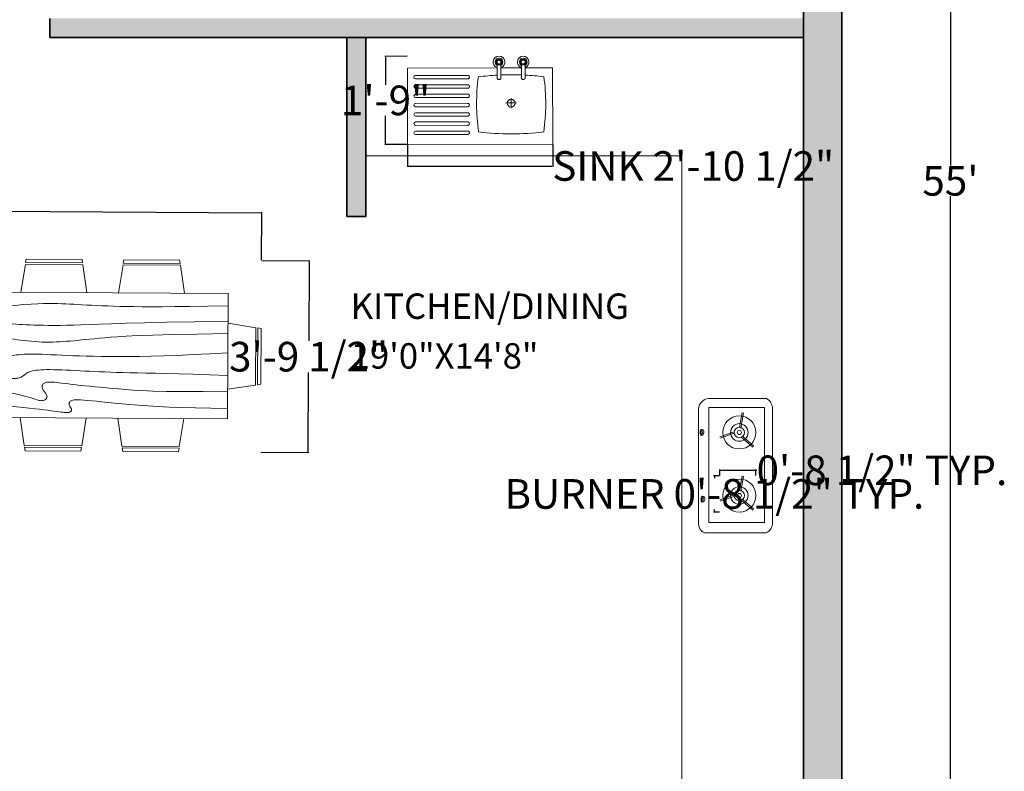
# Model space of a CAD drawing. Units: inches. Extents: x 1319 to 2030, y 219 to 1069.
# Tile 23 of 28: x 1776 to 2008, y 486 to 663. Entities that reach past the tile are written whole.
import ezdxf

# ---------------------------------------------------------------- set-up
doc = ezdxf.new("R2010")
doc.units = ezdxf.units.IN
doc.header["$MEASUREMENT"] = 0
doc.layers.get('0').update_dxf_attribs({"color": 12})
for name, color, linetype, lineweight in [('A-ANNO-DIMS', 2, 'Continuous', 18), ('A-AREA-IDEN', 250, 'Continuous', 18), ('A-EQPM', 8, 'Continuous', 18), ('A-FLOR-CASE', 8, 'Continuous', 18), ('A-WALL-PATT', 252, 'Continuous', 13), ('C-PROP', 7, 'Continuous', 35), ('furniture', 250, 'Continuous', 18), ('PLUMBING FIXTURES', 252, 'Continuous', 18), ('walls', 250, 'Continuous', 35)]:
    doc.layers.add(name, color=color, linetype=linetype, lineweight=lineweight)
doc.styles.get("Standard").update_dxf_attribs({"font": 'arial.ttf'})
doc.dimstyles.get("Standard").update_dxf_attribs({"dimtxt": 7, "dimasz": 0.18, "dimexe": 0.18, "dimexo": 0.0625, "dimgap": 0.09, "dimtad": 0, "dimtih": 1, "dimtoh": 1, "dimzin": 0, "dimdsep": 46, "dimlunit": 3, "dimtxsty": 'Standard', "dimcen": 0.09, "dimadec": 0, "dimazin": 0, "dimtfac": 1, "dimtofl": 0, "dimtmove": 0, "dimatfit": 3, "dimfxl": 1, "dimtolj": 1, "dimtzin": 0, "dimarcsym": 0})

# ---------------------------------------------------------------- blocks, each defined once
blk = doc.blocks.new('Dining Set - 36 x 72 in.')
for p, q in [((-22.2343, 26.00059), (-23.4847, 17.99762)), ((-22.2304, 26), (-5.7608, 26)), ((-22, 27.5), (-22.1562, 26.50042)), ((-5.8416, 26.5), (-22.1534, 26.5)), ((-22, 27.5), (-6, 27.5)), ((-5.8437, 26.49966), (-6, 27.5)), ((-4.5152, 17.99762), (-5.7655, 25.99926)), ((5.7657, 26.00059), (4.5153, 17.99762)), ((5.7696, 26), (22.2392, 26)), ((6, 27.5), (5.8438, 26.50042)), ((22.1584, 26.5), (5.8466, 26.5)), ((6, 27.5), (22, 27.5)), ((22.1563, 26.49966), (22, 27.5)), ((23.4848, 17.99762), (22.2345, 25.99926)), ((36, 18), (-36, 18)), ((-36, 18), (-36, -18)), ((36, -18), (36, 18)), ((-44.0006, 8.23428), (-35.9976, 9.48474)), ((44.0006, 8.23428), (35.9976, 9.48474)), ((-45.5, 8), (-44.5004, 8.15617)), ((-45.5, 8), (-45.5, -8)), ((-44.5, -8.15843), (-44.5, 8.15338)), ((-44, 8.23041), (-44, -8.23915)), ((44, 8.23041), (44, -8.23915)), ((44.5, -8.15843), (44.5, 8.15338)), ((45.5, 8), (44.5005, 8.15617)), ((45.5, 8), (45.5, -8)), ((-44.4997, -8.15631), (-45.5, -8)), ((-35.9976, -9.48476), (-43.9993, -8.2345)), ((35.9976, -9.48476), (43.9993, -8.2345)), ((44.4997, -8.15631), (45.5, -8)), ((-36, -18), (36, -18)), ((-22.2343, -26.0006), (-23.4847, -17.99762)), ((-4.5152, -17.99762), (-5.7655, -25.99928)), ((5.7657, -26.0006), (4.5153, -17.99762)), ((23.4848, -17.99762), (22.2345, -25.99928)), ((-22.2304, -26), (-5.7608, -26)), ((-22, -27.5), (-22.1562, -26.50044)), ((-5.8416, -26.5), (-22.1534, -26.5)), ((-22, -27.5), (-6, -27.5)), ((-5.8437, -26.49967), (-6, -27.5)), ((5.7696, -26), (22.2392, -26)), ((6, -27.5), (5.8438, -26.50044)), ((22.1584, -26.5), (5.8466, -26.5)), ((6, -27.5), (22, -27.5)), ((22.1563, -26.49967), (22, -27.5))]:
    blk.add_line(p, q)
for points in [[(-36, 15), (-31.1772, 14.97754), (-26.8079, 14.91406), (-22.8538, 14.81543), (-19.276, 14.6875), (-16.0362, 14.53613), (-13.0957, 14.36718), (-10.4159, 14.18652), (-7.9583, 14), (-5.6904, 13.81315), (-3.6035, 13.63021), (-1.6954, 13.45508), (0.0365, 13.29166), (1.5945, 13.14388), (2.9811, 13.01562), (4.1988, 12.9108), (5.25, 12.83333), (6.1393, 12.78613), (6.8802, 12.76823), (7.4883, 12.77767), (7.9792, 12.8125), (8.3685, 12.87077), (8.6719, 12.95052), (8.9049, 13.0498), (9.0833, 13.16666), (9.2205, 13.29899), (9.3216, 13.44401), (9.3895, 13.59879), (9.4271, 13.76041), (9.4373, 13.92594), (9.4232, 14.09245), (9.3875, 14.257), (9.3333, 14.41666), (9.2638, 14.56917), (9.1836, 14.71484), (9.0975, 14.85465), (9.0104, 14.98958), (8.9272, 15.1206), (8.8529, 15.2487), (8.7922, 15.37483), (8.75, 15.5), (8.7305, 15.62467), (8.7344, 15.74739), (8.7617, 15.86621), (8.8125, 15.97916), (8.8867, 16.08431), (8.9844, 16.17968), (9.1055, 16.26334), (9.25, 16.33333), (9.4189, 16.38802), (9.6172, 16.42708), (9.8506, 16.45052), (10.125, 16.45833), (10.4463, 16.45052), (10.8203, 16.42708), (11.2529, 16.38802), (11.75, 16.33333), (12.3184, 16.26318), (12.9694, 16.17838), (13.7151, 16.07991), (14.5677, 15.96875), (15.5395, 15.84586), (16.6426, 15.71224), (17.8893, 15.56884), (19.2917, 15.41666), (20.859, 15.25667), (22.5879, 15.08984), (24.4721, 14.91715), (26.5052, 14.73958), (28.6809, 14.5581), (30.9929, 14.3737), (33.4347, 14.18733), (36, 14)], [(-36, 10), (-28.9766, 10.14274), (-23.1725, 10.20442), (-18.4241, 10.19775), (-14.5677, 10.13541), (-11.4399, 10.03011), (-8.877, 9.89453), (-6.7154, 9.74137), (-4.7917, 9.58333), (-2.9698, 9.43082), (-1.2246, 9.28515), (0.4415, 9.14534), (2.026, 9.01041), (3.5266, 8.87939), (4.9408, 8.7513), (6.266, 8.62516), (7.5, 8.5), (8.6411, 8.37549), (9.6914, 8.2539), (10.6538, 8.13818), (11.5312, 8.03125), (12.3267, 7.93603), (13.043, 7.85547), (13.6831, 7.79248), (14.25, 7.75), (14.7471, 7.7303), (15.1797, 7.73307), (15.5537, 7.75732), (15.875, 7.80208), (16.1494, 7.86637), (16.3828, 7.94922), (16.5811, 8.04964), (16.75, 8.16666), (16.8944, 8.29915), (17.0143, 8.44531), (17.1089, 8.60319), (17.1771, 8.77083), (17.218, 8.94629), (17.2305, 9.1276), (17.2137, 9.31282), (17.1667, 9.5), (17.0895, 9.6875), (16.987, 9.875), (16.8649, 10.0625), (16.7292, 10.25), (16.5856, 10.4375), (16.4401, 10.625), (16.2985, 10.8125), (16.1667, 11), (16.05, 11.18733), (15.9518, 11.3737), (15.8752, 11.5581), (15.8229, 11.73958), (15.798, 11.91715), (15.8034, 12.08984), (15.842, 12.25667), (15.9167, 12.41666), (16.0295, 12.56836), (16.1784, 12.70833), (16.3605, 12.83268), (16.5729, 12.9375), (16.8127, 13.01888), (17.0768, 13.07291), (17.3625, 13.0957), (17.6667, 13.08333), (17.9894, 13.03312), (18.3418, 12.94726), (18.7382, 12.82918), (19.1927, 12.68229), (19.7195, 12.51001), (20.3327, 12.31575), (21.0465, 12.10294), (21.875, 11.875), (22.8357, 11.63354), (23.959, 11.37304), (25.2786, 11.08618), (26.8282, 10.76562), (28.6414, 10.40405), (30.752, 9.99414), (33.1936, 9.52856), (36, 9)], [(-36, 5.5), (-30.7157, 5.3348), (-26.069, 5.20963), (-21.9946, 5.11767), (-18.4271, 5.05208), (-15.3009, 5.00602), (-12.5508, 4.97265), (-10.1112, 4.94515), (-7.9167, 4.91666), (-5.909, 4.88167), (-4.0586, 4.83984), (-2.3429, 4.79215), (-0.7396, 4.73958), (0.7739, 4.6831), (2.22, 4.6237), (3.6213, 4.56233), (5, 4.5), (6.373, 4.43782), (7.7344, 4.3776), (9.0723, 4.32129), (10.375, 4.27083), (11.6309, 4.22819), (12.8281, 4.19531), (13.9551, 4.17415), (15, 4.16666), (15.954, 4.17448), (16.819, 4.19791), (17.6001, 4.23698), (18.3021, 4.29166), (18.9299, 4.36198), (19.4883, 4.44791), (19.9823, 4.54948), (20.4167, 4.66666), (20.7969, 4.79899), (21.1302, 4.94401), (21.4245, 5.09879), (21.6875, 5.26041), (21.9271, 5.42594), (22.1511, 5.59245), (22.3672, 5.757), (22.5834, 5.91666), (22.8065, 6.06868), (23.0404, 6.21093), (23.2879, 6.34147), (23.5521, 6.45833), (23.8358, 6.55957), (24.142, 6.64323), (24.4735, 6.70735), (24.8334, 6.75), (25.2235, 6.76969), (25.642, 6.76692), (26.0858, 6.74267), (26.5521, 6.69791), (27.0379, 6.63362), (27.5404, 6.55078), (28.0565, 6.45036), (28.5834, 6.33333), (29.1242, 6.19987), (29.7071, 6.04687), (30.3661, 5.87044), (31.1354, 5.66666), (32.0493, 5.43164), (33.142, 5.16146), (34.4475, 4.85221), (36, 4.5)], [(-36, -1), (-30.7915, -0.6591), (-26.0195, -0.38216), (-21.6519, -0.16284), (-17.6563, 0.00521), (-14.0005, 0.12833), (-10.6523, 0.21289), (-7.5796, 0.26522), (-4.75, 0.29166), (-2.134, 0.29793), (0.2878, 0.28711), (2.5317, 0.26163), (4.6146, 0.22396), (6.5529, 0.17651), (8.3633, 0.12174), (10.0623, 0.06209), (11.6667, 0), (13.1899, -0.06201), (14.6341, -0.1211), (15.9982, -0.17432), (17.2813, -0.21875), (18.4823, -0.25147), (19.6003, -0.26953), (20.6343, -0.27002), (21.5834, -0.25), (22.4481, -0.20768), (23.2357, -0.14584), (23.9549, -0.06836), (24.6146, 0.02083), (25.2235, 0.11784), (25.7904, 0.21875), (26.3241, 0.31966), (26.8334, 0.41666), (27.3265, 0.50618), (27.8099, 0.58593), (28.2894, 0.65397), (28.7709, 0.70833), (29.2601, 0.74707), (29.763, 0.76823), (30.2855, 0.76985), (30.8334, 0.75), (31.4088, 0.70784), (31.9994, 0.64713), (32.589, 0.57275), (33.1615, 0.48958), (33.7008, 0.4025), (34.1908, 0.3164), (34.6153, 0.23616), (34.9584, 0.16666), (35.2099, 0.11165), (35.3848, 0.07031), (35.504, 0.04069), (35.5886, 0.02083), (35.6594, 0.00879), (35.7377, 0.0026), (35.8442, 0.00032), (36, 0)], [(-36, -6.5), (-27.1843, -6.31267), (-20.084, -6.1263), (-14.469, -5.9419), (-10.1094, -5.76042), (-6.7752, -5.58285), (-4.2363, -5.41016), (-2.2629, -5.24333), (-0.625, -5.08334), (0.8708, -4.93099), (2.2715, -4.78646), (3.5872, -4.64974), (4.8281, -4.52084), (6.0046, -4.39974), (7.127, -4.28646), (8.2053, -4.18099), (9.25, -4.08334), (10.2705, -3.99382), (11.2734, -3.91407), (12.2647, -3.84603), (13.25, -3.79167), (14.2354, -3.75293), (15.2266, -3.73177), (16.2295, -3.73015), (17.25, -3.75), (18.2912, -3.79248), (19.3451, -3.85547), (20.4009, -3.93604), (21.4479, -4.03125), (22.4754, -4.13819), (23.4727, -4.25391), (24.4289, -4.37549), (25.3334, -4.5), (26.1785, -4.62492), (26.9694, -4.74935), (27.7145, -4.87281), (28.4219, -4.99479), (29.1, -5.11483), (29.7572, -5.23242), (30.4016, -5.34709), (31.0417, -5.45834), (31.6837, -5.56437), (32.3262, -5.65821), (32.9658, -5.73153), (33.599, -5.77604), (34.2224, -5.78345), (34.8327, -5.74545), (35.4264, -5.65373), (36, -5.5)], [(-36, -10), (-26.4022, -9.81299), (-18.4675, -9.62891), (-11.9839, -9.45069), (-6.7396, -9.28125), (-2.5226, -9.12354), (0.8789, -8.98047), (3.6769, -8.85498), (6.0833, -8.75), (8.2767, -8.66765), (10.3021, -8.60677), (12.1712, -8.56543), (13.8958, -8.54167), (15.4876, -8.53353), (16.9583, -8.53907), (18.3197, -8.55632), (19.5834, -8.58334), (20.7616, -8.61841), (21.8685, -8.66081), (22.9188, -8.71004), (23.9271, -8.76563), (24.9081, -8.82707), (25.8763, -8.89388), (26.8465, -8.96558), (27.8334, -9.04167), (28.8474, -9.12118), (29.8828, -9.20117), (30.93, -9.27824), (31.9792, -9.34896), (33.0205, -9.40991), (34.0443, -9.45768), (35.0407, -9.48885), (36, -9.5)], [(-36, -14.5), (-30.0881, -14.33513), (-25.0332, -14.21224), (-20.7312, -14.12647), (-17.0781, -14.07292), (-13.97, -14.04671), (-11.3027, -14.04297), (-8.9724, -14.05681), (-6.875, -14.08334), (-4.9224, -14.11833), (-3.0905, -14.16016), (-1.3709, -14.20785), (0.2448, -14.26042), (1.7647, -14.3169), (3.1973, -14.3763), (4.5507, -14.43767), (5.8333, -14.5), (7.0554, -14.5621), (8.235, -14.62175), (9.3922, -14.67652), (10.5469, -14.72396), (11.7192, -14.76164), (12.929, -14.78711), (14.1965, -14.79794), (15.5417, -14.79167), (16.9933, -14.76424), (18.6152, -14.70508), (20.4804, -14.60197), (22.6615, -14.44271), (25.2312, -14.21509), (28.2624, -13.9069), (31.8277, -13.50594), (36, -13)]]:
    blk.add_lwpolyline(points)
blk = doc.blocks.new('dining area')
at = {"layer": 'furniture', "xscale": 0.6659924291999282, "yscale": 0.6659924291999282, "zscale": 0.6659924291999282, "rotation": 90}
blk.add_blockref('Dining Set - 36 x 72 in.', (-0.44, 20.51), dxfattribs=at)
blk = doc.blocks.new('A$C799204C7')
for p, q in [((0, 34.2), (17.99, 34.2)), ((0, 0), (0, 34.2)), ((17.99, 13.08), (17.99, 34.2)), ((2.32, 20.01), (2.32, 32.27)), ((3.13, 20.01), (3.13, 32.27)), ((4.48, 20.01), (4.48, 32.27)), ((5.29, 20.01), (5.29, 32.27)), ((6.64, 20.01), (6.64, 32.27)), ((7.45, 20.01), (7.45, 32.27)), ((8.85, 20.01), (8.85, 32.27)), ((9.66, 20.01), (9.66, 32.27)), ((11.01, 20.01), (11.01, 32.27)), ((11.82, 20.01), (11.82, 32.27)), ((13.22, 20.01), (13.22, 32.27)), ((14.03, 20.01), (14.03, 32.27)), ((15.42, 20.01), (15.42, 32.27)), ((16.24, 20.01), (16.24, 32.27)), ((18.59, 13.08), (15.71, 13.08)), ((15.71, 12.17), (18.59, 12.17)), ((17.99, 7.36), (17.99, 12.17)), ((8.52, 9.77), (10.9, 9.77)), ((9.73, 11), (9.73, 8.54)), ((18.59, 7.36), (15.71, 7.36)), ((15.71, 6.45), (18.59, 6.45)), ((17.99, 0), (17.99, 6.45)), ((0, 0), (17.99, 0))]:
    blk.add_line(p, q)
for centre, radius in [((19.38, 12.62), 0.684), ((19.38, 12.62), 0.456), ((9.7, 9.77), 0.916), ((19.38, 6.91), 0.684), ((19.38, 6.91), 0.456)]:
    blk.add_circle(centre, radius)
for centre, radius, start, end in [((2.72, 32.27), 0.407, 0, 180), ((4.88, 32.27), 0.407, 0, 180), ((7.05, 32.27), 0.407, 0, 180), ((9.25, 32.27), 0.407, 0, 180), ((11.42, 32.27), 0.407, 0, 180), ((13.62, 32.27), 0.407, 0, 180), ((15.83, 32.27), 0.407, 0, 180), ((2.72, 20.01), 0.407, 180, 0), ((4.88, 20.01), 0.407, 180, 0), ((7.05, 20.01), 0.407, 180, 0), ((9.25, 20.01), 0.407, 180, 0), ((11.42, 20.01), 0.407, 180, 0), ((13.62, 20.01), 0.407, 180, 0), ((15.83, 20.01), 0.407, 180, 0), ((67.33, 9.77), 64.88, 173.1952, 186.8048), ((9.53, -30.19), 48.1, 82.3437, 97.8966), ((-48.51, 9.77), 64.88, 2.9208, 6.8048), ((19.38, 12.62), 1.37, 199.6514, 160.3603), ((15.71, 12.62), 0.456, 90, 270), ((-48.51, 9.77), 64.88, 357.8723, 2.115), ((19.38, 12.62), 0.911, 210.3431, 149.7554), ((15.71, 6.91), 0.456, 90, 270), ((19.38, 6.91), 1.37, 199.6514, 160.3603), ((19.38, 6.91), 0.911, 210.3431, 149.7554), ((-48.51, 9.77), 64.88, 353.1952, 357.0665), ((9.53, 49.73), 48.1, 262.1034, 277.6563)]:
    blk.add_arc(centre, radius, start, end)
blk = doc.blocks.new('sink')
at = {"layer": 'furniture'}
for p, q in [((8718164202.684322, -1433730581.131674), (8718164202.684322, -1433730583.598095)), ((8718164203.894819, -1433730582.369047), (8718164201.504578, -1433730582.369047)), ((8718164196.150837, -1433730592.638258), (8718164196.150837, -1433730604.938997)), ((8718164196.967728, -1433730592.638258), (8718164196.967728, -1433730604.938997)), ((8718164198.365185, -1433730592.638258), (8718164198.365185, -1433730604.938997)), ((8718164199.182076, -1433730592.638258), (8718164199.182076, -1433730604.938997)), ((8718164200.579533, -1433730592.638258), (8718164200.579533, -1433730604.938997)), ((8718164201.396423, -1433730592.638258), (8718164201.396423, -1433730604.938997)), ((8718164202.748692, -1433730592.638258), (8718164202.748692, -1433730604.938997)), ((8718164203.565582, -1433730592.638258), (8718164203.565582, -1433730604.938997)), ((8718164204.963041, -1433730592.638258), (8718164204.963041, -1433730604.938997)), ((8718164205.779934, -1433730592.638258), (8718164205.779934, -1433730604.938997)), ((8718164207.1322, -1433730592.638258), (8718164207.1322, -1433730604.938997)), ((8718164207.949093, -1433730592.638258), (8718164207.949093, -1433730604.938997)), ((8718164209.301359, -1433730592.638258), (8718164209.301359, -1433730604.938997)), ((8718164210.118252, -1433730592.638258), (8718164210.118252, -1433730604.938997))]:
    blk.add_line(p, q, dxfattribs=at)
for centre, radius in [((8718164192.998869, -1433730579.495552), 0.685789), ((8718164192.998869, -1433730579.495552), 0.457192), ((8718164202.715019, -1433730582.369047), 0.919003), ((8718164192.998869, -1433730585.228166), 0.68579), ((8718164192.998869, -1433730585.228166), 0.68579), ((8718164192.998869, -1433730585.228166), 0.457192)]:
    blk.add_circle(centre, radius, dxfattribs=at)
for centre, radius, start, end in [((8718164196.559284, -1433730592.638258), 0.41045, 354.3355999, 185.6644001), ((8718164198.77363, -1433730592.638258), 0.41045, 354.3355999, 185.6644001), ((8718164200.98798, -1433730592.638258), 0.41045, 354.3355999, 185.6644001), ((8718164203.157139, -1433730592.638258), 0.41045, 354.3355999, 185.6644001), ((8718164205.371487, -1433730592.638258), 0.41045, 354.3355999, 185.6644001), ((8718164207.540646, -1433730592.640262), 0.41045, 354.3355999, 185.6644001), ((8718164209.709805, -1433730592.640262), 0.41045, 354.3355999, 185.6644001), ((8718164196.559284, -1433730604.938997), 0.408445, 180, 0), ((8718164198.77363, -1433730604.938997), 0.408445, 180, 0), ((8718164200.98798, -1433730604.938997), 0.408445, 180, 0), ((8718164203.157139, -1433730604.938997), 0.408445, 180, 0), ((8718164205.371487, -1433730604.938997), 0.408445, 180, 0), ((8718164207.540646, -1433730604.938997), 0.408445, 180, 0), ((8718164209.709805, -1433730604.938997), 0.408445, 180, 0)]:
    blk.add_arc(centre, radius, start, end, dxfattribs=at)
at = {"layer": 'furniture', "xscale": 1.0032, "yscale": 1.0032, "zscale": 1.0032, "rotation": 180}
blk.add_blockref('A$C799204C7', (8718164212.441259, -1433730572.566334), dxfattribs=at)
blk = doc.blocks.new('washbasin')
at = {"layer": 'furniture'}
blk.add_blockref('sink', (-8718164214.119328, 1433730589.721069), dxfattribs=at)
blk = doc.blocks.new('*D29')
at = {"layer": 'A-ANNO-DIMS', "color": 0, "lineweight": -2, "transparency": 16777216}
for p, q in [((1995.58, 955.23), (1995.33, 955.23)), ((1995.51, 955.05), (1995.51, 628.88)), ((1995.51, 295.41), (1995.51, 621.58)), ((1995.58, 295.23), (1995.33, 295.23))]:
    blk.add_line(p, q, dxfattribs=at)
at = {"layer": 'A-ANNO-DIMS', "color": 0, "transparency": 16777216}
for points in [[(1995.48, 955.05), (1995.54, 955.05), (1995.51, 955.23)], [(1995.48, 295.41), (1995.54, 295.41), (1995.51, 295.23)]]:
    blk.add_solid(points, dxfattribs=at)
at = {"layer": 'Defpoints', "color": 0, "transparency": 16777216}
for p in [(1995.64, 955.23), (1995.51, 295.23), (1995.64, 295.23)]:
    blk.add_point(p, dxfattribs=at)
at = {"layer": 'A-ANNO-DIMS', "color": 0, "transparency": 16777216, "insert": (1995.51, 625.23), "char_height": 7, "attachment_point": 5}
blk.add_mtext("\\A1;55'", dxfattribs=at)
blk = doc.blocks.new('COOKTOP-BURNER')
for p, q in [((4.61, 5.14), (5.29, 8.59)), ((4.94, 4.96), (5.59, 8.52)), ((3.4, 4.08), (0, 2.86)), ((3.41, 3.71), (0.09, 2.57)), ((5.08, 2.78), (7.83, 0.44)), ((5.4, 2.97), (8.04, 0.66))]:
    blk.add_line(p, q)
for radius in [3.91, 2.08, 1.22, 0.507]:
    blk.add_circle((4.61, 3.91), radius)
blk = doc.blocks.new('*D50')
at = {"layer": 'A-ANNO-DIMS', "color": 0, "lineweight": -2, "transparency": 16777216}
for p, q in [((1940.98, 555.53), (1939.57, 555.53)), ((1939.75, 555.35), (1939.75, 554.94)), ((1940.98, 546.94), (1939.57, 546.94)), ((1939.75, 547.12), (1939.75, 547.52))]:
    blk.add_line(p, q, dxfattribs=at)
at = {"layer": 'A-ANNO-DIMS', "color": 0, "transparency": 16777216}
for points in [[(1939.72, 555.35), (1939.78, 555.35), (1939.75, 555.53)], [(1939.72, 547.12), (1939.78, 547.12), (1939.75, 546.94)]]:
    blk.add_solid(points, dxfattribs=at)
at = {"layer": 'Defpoints', "color": 0, "transparency": 16777216}
for p in [(1939.75, 555.53), (1941.04, 555.53), (1941.04, 546.94)]:
    blk.add_point(p, dxfattribs=at)
at = {"layer": 'A-ANNO-DIMS', "color": 0, "transparency": 16777216, "insert": (1939.75, 551.23), "char_height": 7, "attachment_point": 5}
blk.add_mtext('\\A1;BURNER 0\'-8 1/2" TYP.', dxfattribs=at)
blk = doc.blocks.new('*D51')
at = {"layer": 'A-ANNO-DIMS', "color": 0, "lineweight": -2, "transparency": 16777216}
for p, q in [((1941.04, 555.59), (1941.04, 556.99)), ((1941.22, 556.81), (1949.39, 556.81)), ((1949.57, 555.59), (1949.57, 556.99)), ((1949.57, 556.81), (1949.75, 556.81))]:
    blk.add_line(p, q, dxfattribs=at)
at = {"layer": 'A-ANNO-DIMS', "color": 0, "transparency": 16777216}
for points in [[(1941.22, 556.84), (1941.22, 556.78), (1941.04, 556.81)], [(1949.39, 556.84), (1949.39, 556.78), (1949.57, 556.81)]]:
    blk.add_solid(points, dxfattribs=at)
at = {"layer": 'Defpoints', "color": 0, "transparency": 16777216}
for p in [(1949.57, 556.81), (1941.04, 555.53), (1949.57, 555.53)]:
    blk.add_point(p, dxfattribs=at)
at = {"layer": 'A-ANNO-DIMS', "color": 0, "transparency": 16777216, "insert": (1979.33, 556.81), "char_height": 7, "attachment_point": 5}
blk.add_mtext('\\A1;0\'-8 1/2" TYP.', dxfattribs=at)
blk = doc.blocks.new('*D54')
at = {"layer": 'A-ANNO-DIMS', "color": 0, "lineweight": -2, "transparency": 16777216}
for p, q in [((1757.94, 618.08), (1757.76, 618.08)), ((1757.87, 606.9), (1757.94, 618.26)), ((1832.71, 617.63), (1758.12, 618.08)), ((1832.82, 606.45), (1832.89, 617.81))]:
    blk.add_line(p, q, dxfattribs=at)
at = {"layer": 'A-ANNO-DIMS', "color": 0, "transparency": 16777216}
for points in [[(1758.12, 618.11), (1758.12, 618.05), (1757.94, 618.08)], [(1832.71, 617.66), (1832.71, 617.6), (1832.89, 617.63)]]:
    blk.add_solid(points, dxfattribs=at)
at = {"layer": 'Defpoints', "color": 0, "transparency": 16777216}
for p in [(1757.94, 618.08), (1757.87, 606.84), (1832.82, 606.38)]:
    blk.add_point(p, dxfattribs=at)
at = {"layer": 'A-ANNO-DIMS', "color": 0, "transparency": 16777216, "insert": (1719.2, 618.08), "char_height": 7, "attachment_point": 5}
blk.add_mtext('\\A1;DINING SET 6\'-3"', dxfattribs=at)
blk = doc.blocks.new('*D55')
at = {"layer": 'A-ANNO-DIMS', "color": 0, "lineweight": -2, "transparency": 16777216}
for p, q in [((1832.88, 606.38), (1844.24, 606.31)), ((1844.06, 606.14), (1843.94, 587.38)), ((1843.78, 561.2), (1843.9, 579.96)), ((1832.6, 561.09), (1843.96, 561.02))]:
    blk.add_line(p, q, dxfattribs=at)
at = {"layer": 'A-ANNO-DIMS', "color": 0, "transparency": 16777216}
for points in [[(1844.03, 606.14), (1844.09, 606.14), (1844.06, 606.32)], [(1843.75, 561.2), (1843.81, 561.2), (1843.78, 561.02)]]:
    blk.add_solid(points, dxfattribs=at)
at = {"layer": 'Defpoints', "color": 0, "transparency": 16777216}
for p in [(1832.82, 606.38), (1844.06, 606.32), (1832.54, 561.09)]:
    blk.add_point(p, dxfattribs=at)
at = {"layer": 'A-ANNO-DIMS', "color": 0, "transparency": 16777216, "insert": (1843.92, 583.67), "char_height": 7, "attachment_point": 5}
blk.add_mtext('\\A1;3\'-9 1/2"', dxfattribs=at)
blk = doc.blocks.new('*D58')
at = {"layer": 'A-ANNO-DIMS', "color": 0, "lineweight": -2, "transparency": 16777216}
for p, q in [((1867.26, 633.79), (1867.26, 628.52)), ((1901.57, 633.82), (1901.57, 628.56)), ((1867.44, 628.7), (1901.39, 628.74)), ((1901.57, 628.74), (1901.75, 628.74))]:
    blk.add_line(p, q, dxfattribs=at)
at = {"layer": 'A-ANNO-DIMS', "color": 0, "transparency": 16777216}
for points in [[(1867.44, 628.73), (1867.44, 628.67), (1867.26, 628.7)], [(1901.39, 628.77), (1901.39, 628.71), (1901.57, 628.74)]]:
    blk.add_solid(points, dxfattribs=at)
at = {"layer": 'Defpoints', "color": 0, "transparency": 16777216}
for p in [(1867.26, 633.85), (1901.57, 633.88), (1901.57, 628.74)]:
    blk.add_point(p, dxfattribs=at)
at = {"layer": 'A-ANNO-DIMS', "color": 0, "transparency": 16777216, "insert": (1934.77, 628.74), "char_height": 7, "attachment_point": 5}
blk.add_mtext('\\A1;SINK 2\'-10 1/2"', dxfattribs=at)
blk = doc.blocks.new('*D59')
at = {"layer": 'A-ANNO-DIMS', "color": 0, "lineweight": -2, "transparency": 16777216}
for p, q in [((1867.18, 654.67), (1861.91, 654.66)), ((1862.09, 654.48), (1862.1, 647.92)), ((1862.11, 634.03), (1862.1, 640.59)), ((1867.19, 633.85), (1861.93, 633.85))]:
    blk.add_line(p, q, dxfattribs=at)
at = {"layer": 'A-ANNO-DIMS', "color": 0, "transparency": 16777216}
for points in [[(1862.12, 654.48), (1862.06, 654.48), (1862.09, 654.66)], [(1862.14, 634.03), (1862.08, 634.03), (1862.11, 633.85)]]:
    blk.add_solid(points, dxfattribs=at)
at = {"layer": 'Defpoints', "color": 0, "transparency": 16777216}
for p in [(1867.24, 654.67), (1862.11, 633.85), (1867.26, 633.85)]:
    blk.add_point(p, dxfattribs=at)
at = {"layer": 'A-ANNO-DIMS', "color": 0, "transparency": 16777216, "insert": (1862.1, 644.25), "char_height": 7, "attachment_point": 5}
blk.add_mtext('\\A1;1\'-9"', dxfattribs=at)

msp = doc.modelspace()

# ---------------------------------------------------------------- hatches: boundary and pattern name
at = {"layer": 'A-WALL-PATT'}
h = msp.add_hatch(color=256, dxfattribs=at)
h.dxf.hatch_style = 1
h.paths.add_polyline_path([(1378.843, 946.227), (1960.843, 946.227), (1960.843, 860.616), (1922.194, 860.616), (1922.194, 851.616), (1960.843, 851.616), (1960.843, 304.227), (1578.343, 304.227), (1578.343, 295.227), (1969.843, 295.227), (1969.843, 955.227), (1369.843, 955.227), (1369.843, 295.227), (1378.843, 295.227)])
h = msp.add_hatch(color=256, dxfattribs=at)
h.dxf.hatch_style = 1
h.paths.add_polyline_path([(1856.292, 860.616), (1812.343, 860.616), (1812.343, 851.616), (1812.343, 700.993), (1816.843, 700.993), (1816.843, 851.616), (1856.292, 851.616)])
h.paths.add_polyline_path([(1960.843, 663.616), (1812.343, 663.616), (1782.783, 663.616), (1782.783, 659.116), (1812.343, 659.116), (1960.843, 659.116)])
h.paths.add_polyline_path([(1857.424, 659.116), (1852.924, 659.116), (1852.924, 616.807), (1857.424, 616.807)])
h.paths.add_polyline_path([(1735.843, 661.727), (1731.843, 661.727), (1636.133, 661.727), (1636.133, 657.227), (1731.343, 657.227), (1731.343, 481.227), (1618.616, 481.227), (1618.616, 472.227), (1639.343, 472.227), (1639.343, 384.227), (1627.044, 384.227), (1627.044, 375.227), (1648.343, 375.227), (1648.343, 384.227), (1648.343, 472.227), (1750.706, 472.227), (1750.706, 481.227), (1735.843, 481.227), (1735.843, 657.727)])
h.paths.add_polyline_path([(1587.343, 481.227), (1578.343, 481.227), (1578.343, 375.227), (1597.622, 375.227), (1597.622, 384.227), (1587.343, 384.227)])
h.paths.add_polyline_path([(1769.593, 384.227), (1693.482, 384.227), (1693.482, 375.227), (1769.593, 375.227)])
h.paths.add_polyline_path([(1775.828, 481.227), (1765.831, 481.227), (1765.831, 472.227), (1775.828, 472.227)])
h.paths.add_polyline_path([(1824.625, 481.227), (1820.343, 481.227), (1820.343, 476.727), (1824.625, 476.727), (1824.625, 477.545)], flags=0)
h.paths.add_polyline_path([(1896.843, 481.227), (1852.26, 481.227), (1852.26, 476.727), (1892.343, 476.727), (1892.343, 384.227), (1881.742, 384.227), (1881.742, 375.227), (1913.435, 375.227), (1913.435, 384.227), (1896.843, 384.227)])
h.paths.add_polyline_path([(1960.843, 481.227), (1931.341, 481.227), (1931.341, 476.727), (1960.843, 476.727)])
h.paths.add_polyline_path([(1736.343, 918.227), (1731.843, 918.227), (1731.843, 890.227), (1582.843, 890.227), (1582.843, 781.727), (1582.843, 769.171), (1587.343, 769.171), (1587.343, 781.727), (1587.343, 885.727), (1731.843, 885.727), (1731.843, 851.616), (1736.343, 851.616), (1736.343, 890.227)])
h.paths.add_polyline_path([(1781.022, 860.616), (1773.021, 860.616, -0.0322281), (1773.289, 856.464), (1773.289, 851.616), (1781.022, 851.616)])
h.paths.add_polyline_path([(1587.343, 946.227), (1582.843, 946.227), (1582.843, 926.136), (1587.343, 926.136)])
h.paths.add_polyline_path([(1647.843, 946.227), (1643.343, 946.227), (1643.343, 926.136), (1647.843, 926.136)])
h.paths.add_polyline_path([(1543.343, 786.227), (1429.843, 786.227), (1429.843, 757.555), (1434.343, 757.555), (1438.843, 757.555), (1438.843, 781.727), (1543.343, 781.727)])
h.paths.add_polyline_path([(1543.343, 781.727), (1538.843, 781.727), (1538.843, 709.727), (1534.597, 709.727), (1534.597, 705.227), (1543.343, 705.227), (1543.343, 709.727)])
h.paths.add_polyline_path([(1499.955, 709.727), (1438.843, 709.727), (1438.843, 734.463), (1429.843, 734.463), (1429.843, 552.227), (1470.241, 552.227), (1470.241, 561.227), (1438.843, 561.227), (1438.843, 705.227), (1499.955, 705.227)])
h.paths.add_polyline_path([(1587.343, 709.727), (1582.843, 709.727), (1582.843, 561.227), (1543.433, 561.227), (1543.433, 552.227), (1587.343, 552.227)])
h.paths.add_polyline_path([(1546.835, 709.727), (1543.343, 709.727), (1543.343, 705.227), (1546.835, 705.227)])
h.paths.add_polyline_path([(1582.843, 709.727), (1579.15, 709.727), (1579.15, 705.227), (1582.843, 705.227)], flags=17)
h.paths.add_polyline_path([(1548.368, 786.227), (1543.343, 786.227), (1543.343, 781.727), (1548.368, 781.727)])
h.paths.add_polyline_path([(1582.843, 786.227), (1580.683, 786.227), (1580.683, 781.727), (1582.843, 781.727)])
h.paths.add_polyline_path([(1587.343, 892.402), (1582.843, 892.402), (1582.843, 890.227), (1587.343, 890.227)], flags=17)
h.paths.add_polyline_path([(1647.843, 892.402), (1643.343, 892.402), (1643.343, 890.227), (1647.843, 890.227)], flags=17)
h.paths.add_polyline_path([(1740.974, 856.464), (1740.974, 860.616), (1736.343, 860.616), (1736.343, 851.616), (1740.974, 851.616)])
h.paths.add_polyline_path([(1853.989, 384.227), (1820.343, 384.227), (1820.343, 402.924), (1815.843, 402.924), (1815.843, 375.227), (1853.989, 375.227)])
h.paths.add_polyline_path([(1892.343, 436.227), (1820.343, 436.227), (1820.343, 481.227), (1815.843, 481.227), (1815.843, 431.727), (1892.343, 431.727)])
h.paths.add_polyline_path([(1849.175, 481.227), (1824.625, 481.227), (1824.625, 477.545), (1825.699, 477.545), (1825.699, 453.018, 0.4014527), (1849.175, 477.545)], flags=0)
h.paths.add_polyline_path([(1960.843, 384.227), (1941.188, 384.227), (1941.188, 375.227), (1960.843, 375.227)])
h.paths.add_polyline_path([(1902.267, 481.227), (1896.843, 481.227), (1896.843, 476.727), (1902.267, 476.727), (1902.267, 477.44)], flags=0)

# ---------------------------------------------------------------- linework, layer by layer
at = {"layer": 'A-EQPM'}
for p, q in [((1952.047, 573.783), (1938.425, 573.783)), ((1936.031, 570.707), (1936.031, 544.47)), ((1951.565, 571.642), (1938.425, 571.642)), ((1938.425, 571.642), (1938.425, 544.47)), ((1951.565, 544.47), (1951.565, 571.642)), ((1953.45, 571.642), (1953.45, 544.47)), ((1938.425, 544.47), (1951.565, 544.47)), ((1951.973, 542.023), (1937.437, 542.023))]:
    msp.add_line(p, q, dxfattribs=at)
for centre, radius, start, end in [((1938.604, 571.174), 2.615, 93.92707, 190.30452), ((1950.841, 571.463), 2.615, 3.92707, 62.5308), ((1938.421, 544.216), 2.404, 173.93636, 246.89401), ((1951.056, 544.245), 2.404, 292.40616, 5.36382)]:
    msp.add_arc(centre, radius, start, end, dxfattribs=at)
for centre, major_axis, ratio in [((1936.652, 565.767), (0.02, 0.713), 0.3769734), ((1936.921, 565.759), (0.043, 0.664), 0.4928397), ((1936.879, 549.997), (0.02, 0.713), 0.3769734), ((1937.148, 549.989), (0.043, 0.664), 0.4928397)]:
    msp.add_ellipse(centre, major_axis=major_axis, ratio=ratio, dxfattribs=at)
at = {"layer": 'A-FLOR-CASE'}
for p, q in [((1857.424, 631.139), (1932.091, 631.139)), ((1932.091, 631.139), (1932.091, 481.227))]:
    msp.add_line(p, q, dxfattribs=at)
at = {"layer": 'C-PROP'}
msp.add_line((1969.843, 955.227), (1969.843, 295.227), dxfattribs=at)
at = {"layer": 'walls'}
for p, q in [((1960.843, 851.616), (1960.843, 304.227)), ((1782.783, 663.616), (1782.783, 659.116)), ((1782.783, 659.116), (1812.343, 659.116)), ((1812.343, 659.116), (1960.843, 659.116)), ((1852.924, 659.116), (1852.924, 616.807)), ((1857.424, 616.807), (1857.424, 659.116)), ((1852.924, 616.807), (1857.424, 616.807))]:
    msp.add_line(p, q, dxfattribs=at)

# ---------------------------------------------------------------- block references
at = {"layer": 'A-EQPM'}
for p in [(1941.042, 561.851), (1941.042, 546.938)]:
    msp.add_blockref('COOKTOP-BURNER', p, dxfattribs=at)
at = {"layer": 'furniture', "xscale": 1.236602255742101, "yscale": 1.236602255742101, "zscale": 1.236602255742101, "rotation": 89.64970471612386}
msp.add_blockref('dining area', (1820.569, 584.353), dxfattribs=at)
at = {"layer": 'PLUMBING FIXTURES', "rotation": 270.052267437799}
msp.add_blockref('washbasin', (1884.413, 632.189), dxfattribs=at)

# ---------------------------------------------------------------- texts
at = {"layer": 'A-AREA-IDEN'}
for s, p in [('KITCHEN/DINING', (1853.848, 592.602)), ('19\'0"X14\'8"', (1853.848, 580.853))]:
    msp.add_text(s, height=6.01124, dxfattribs=at).set_placement(p)

# ---------------------------------------------------------------- dimensions: what is measured, and where the dimension line sits
at = {"layer": 'A-ANNO-DIMS'}
for base, p1, p2, angle, override, picture, middle in [((1995.506, 295.227), (1995.643, 955.227), (1995.643, 295.227), 90, {"dimclrd": 0, "dimclre": 0, "dimclrt": 0}, '*D29', (1995.506, 625.227)), ((1862.11, 633.846), (1867.238, 654.665), (1867.257, 633.851), 270.05227, {"dimdec": 1, "dimlfac": 1, "dimrnd": 0, "dimzin": 1, "dimdsep": 46, "dimlunit": 4, "dimfrac": 2}, '*D59', (1862.101, 644.253)), ((1844.059, 606.315), (1832.541, 561.089), (1832.818, 606.384), 89.6497, {"dimdec": 1, "dimlfac": 1, "dimrnd": 0, "dimzin": 1, "dimdsep": 46, "dimlunit": 4, "dimfrac": 2}, '*D55', (1843.921, 583.668))]:
    dim = msp.add_linear_dim(base=base, p1=p1, p2=p2, angle=angle, dimstyle='Standard', override=override, dxfattribs=at)
    dim.commit()
    dim.dimension.update_dxf_attribs({"geometry": picture, "text_midpoint": middle})
for base, p1, p2, angle, text, picture, middle in [((1901.571, 628.736), (1867.257, 633.851), (1901.566, 633.882), 0.05227, 'SINK <>', '*D58', (1934.773, 628.736)), ((1757.943, 618.084), (1832.818, 606.384), (1757.874, 606.842), 179.6497, 'DINING SET <>', '*D54', (1719.204, 618.085)), ((1939.754, 555.525), (1941.042, 546.938), (1941.042, 555.525), 90, 'BURNER <> TYP.', '*D50', (1939.754, 551.231))]:
    dim = msp.add_linear_dim(base=base, p1=p1, p2=p2, angle=angle, text=text, dimstyle='Standard', override={"dimdec": 1, "dimlfac": 1, "dimrnd": 0, "dimzin": 1, "dimdsep": 46, "dimlunit": 4, "dimfrac": 2}, dxfattribs=at)
    dim.commit()
    dim.dimension.update_dxf_attribs({"geometry": picture, "text_midpoint": middle})
dim = msp.add_linear_dim(base=(1949.569, 556.813), p1=(1941.042, 555.525), p2=(1949.569, 555.525), text='<> TYP.', dimstyle='Standard', override={"dimdec": 1, "dimlfac": 1, "dimrnd": 0, "dimzin": 1, "dimdsep": 46, "dimlunit": 4, "dimfrac": 2}, dxfattribs=at)
dim.commit()
dim.dimension.update_dxf_attribs({"geometry": '*D51', "text_midpoint": (1979.329, 556.813)})

doc.saveas('drawing.dxf')
